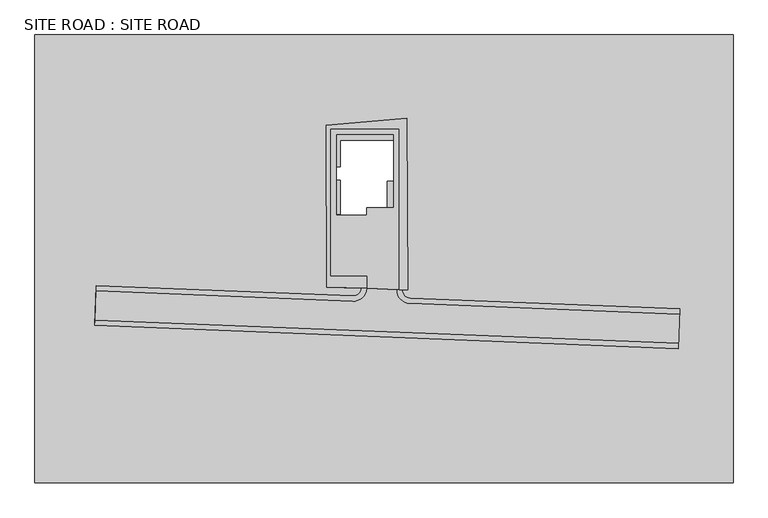
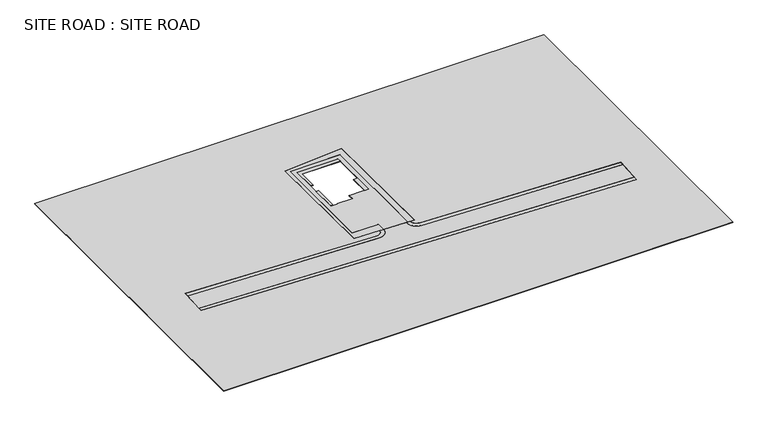
"""IFC4 building model written with IfcOpenShell, lengths in millimetres: proxy geometry, SITE ROAD : SITE ROAD."""

from ifc_helpers import new_model, si_unit, point, frame, frame_2d, origin, origin_with_axes, place, context, project, spatial, polyline, circle_curve, trimmed, segment, composite_curve, outline, extrude, source, transform, mapped, element, save


def site_road_site_road_cda8f1bc(model_context):
    return source(origin(), model_context, "Body", "SweptSolid", [
        extrude(outline(composite_curve([segment(polyline([(-5323.4846863, -24160.3398157), (379.8530763, -24364.5268641)]), True, "CONTINUOUS"), segment(trimmed(circle_curve(frame_2d((2878.0993081, -24458.1525289)), 2500.0), [point((379.8530763, -24364.5268641))], [point((2778.0134737, -26956.1482907))], True, "CARTESIAN"), True, "CONTINUOUS"), segment(polyline([(2778.0134737, -26956.1482907), (53419.5551039, -28985.1753319), (53193.7504784, -34479.8199844), (-56289.5137381, -30093.2137218), (-56064.839832, -24626.0835674), (-7921.4347509, -26555.0191334)]), True, "CONTINUOUS"), segment(trimmed(circle_curve(frame_2d((-7821.3489165, -24057.0233717)), 2500.0), [point((-7921.4347509, -26555.0191334))], [point((-5323.4846863, -24160.3398157))], True, "CARTESIAN"), True, "CONTINUOUS")], self_intersect=False)), origin_with_axes(), (0.0, 0.0, 1.0), 75.0),
        extrude(outline(polyline([(-10908.8712297, -3817.0014262), (-10308.8712297, -3817.0014262), (-10308.8712297, -10267.0014262), (-10908.8712297, -10267.0014262), (-10908.8712297, -3817.0014262)])), origin_with_axes(), (0.0, 0.0, 1.0), 100.0),
        extrude(outline(polyline([(-358.8712297, -4047.0014262), (-358.8712297, -8877.0014262), (-1448.8712297, -8877.0014262), (-1448.8712297, -4047.0014262), (-358.8712297, -4047.0014262)])), origin_with_axes(), (0.0, 0.0, 1.0), 100.0),
        extrude(outline(polyline([(-358.8712297, 3642.9985738), (-10308.8712297, 3642.9985738), (-10308.8712297, -1317.0014262), (-10908.8712297, -1317.0014262), (-10908.8712297, 4642.9985738), (-358.8712297, 4642.9985738), (-358.8712297, 3642.9985738)])), origin_with_axes(), (0.0, 0.0, 1.0), 100.0),
        extrude(outline(polyline([(-12108.8712297, 5842.9985738), (-12108.8712297, -21842.3863739), (-5323.4846863, -21842.3863739), (-5323.4846863, -24160.3398157), (-12818.4447396, -23892.0103155), (-12941.7553777, 6437.7390155), (2241.41409, 7752.6401203), (2409.7426273, -24437.1995995), (841.1287703, -24381.0411451), (841.1287703, 5842.9985738), (-12108.8712297, 5842.9985738)])), origin_with_axes(), (0.0, 0.0, 1.0), 100.0),
        extrude(outline(polyline([(63434.9499784, 23414.0184336), (63434.9499784, -60585.9815664), (-67565.0500216, -60585.9815664), (-67565.0500216, 23414.0184336), (63434.9499784, 23414.0184336)]), holes=[composite_curve([segment(polyline([(-12941.7553777, 6437.7390155), (-12818.4232308, -23897.3006555), (-6323.0723485, -24129.8428229)]), True, "CONTINUOUS"), segment(trimmed(circle_curve(frame_2d((-7821.6488643, -24064.5096292)), 1500.0), [point((-6323.0723485, -24129.8428229))], [point((-7881.7003649, -25563.3070863))], False, "CARTESIAN"), True, "CONTINUOUS"), segment(polyline([(-7881.7003649, -25563.3070863), (-56024.0812791, -23634.412555), (-56330.7861339, -31097.6528943), (53152.4780827, -35484.2591569), (53460.3136567, -27993.5043195), (2817.7478597, -25964.4362435)]), True, "CONTINUOUS"), segment(trimmed(circle_curve(frame_2d((2877.7993603, -24465.6387865)), 1500.0), [point((2817.7478597, -25964.4362435))], [point((1379.0019032, -24405.5872858))], False, "CARTESIAN"), True, "CONTINUOUS"), segment(polyline([(1379.0019032, -24405.5872858), (2409.7702929, -24442.4901599), (2241.41409, 7752.6401203), (-12941.7553777, 6437.7390155)]), True, "CONTINUOUS")], self_intersect=False)]), origin_with_axes(), (0.0, 0.0, 1.0), 125.0),
        extrude(outline(composite_curve([segment(polyline([(-26956.1482907, 2778.0134737), (-28985.1753319, 53419.5551039), (-27988.2223262, 53460.5252875), (-25959.1542503, 2817.9594904)]), True, "CONTINUOUS"), segment(trimmed(circle_curve(frame_2d((-24460.3567932, 2878.010991)), 1500.0), [point((-25959.1542503, 2817.9594904))], [point((-24400.3052926, 1379.213534))], True, "CARTESIAN"), True, "CONTINUOUS"), segment(polyline([(-24400.3052926, 1379.213534), (-24405.5872858, 1379.0019032), (-24364.5268641, 379.8530763)]), True, "CONTINUOUS"), segment(trimmed(circle_curve(frame_2d((-24458.1525289, 2878.0993081)), 2500.0), [point((-24364.5268641, 379.8530763))], [point((-26956.1482907, 2778.0134737))], False, "CARTESIAN"), True, "CONTINUOUS")], self_intersect=False)), frame((0.0, 0.0, 80.0), z_axis=(0.0, 0.0, -1.0), x_axis=(0.0, 1.0, 0.0)), (0.0, 0.0, 1.0), 80.0),
        extrude(outline(polyline([(53193.7504784, -34479.8199844), (53152.6897134, -35478.9771636), (-56330.5745031, -31092.3709011), (-56289.5137381, -30093.2137218), (53193.7504784, -34479.8199844)])), origin_with_axes(), (0.0, 0.0, 1.0), 80.0),
        extrude(outline(composite_curve([segment(polyline([(-56064.839832, -24626.0835674), (-56023.8696484, -23629.1305617), (-7881.4887342, -25558.025093)]), True, "CONTINUOUS"), segment(trimmed(circle_curve(frame_2d((-7821.4372335, -24059.2276359)), 1500.0), [point((-7881.4887342, -25558.025093))], [point((-6322.6397765, -24119.2791366))], True, "CARTESIAN"), True, "CONTINUOUS"), segment(polyline([(-6322.6397765, -24119.2791366), (-5323.4846863, -24160.3398157)]), True, "CONTINUOUS"), segment(trimmed(circle_curve(frame_2d((-7821.3489165, -24057.0233717)), 2500.0), [point((-5323.4846863, -24160.3398157))], [point((-7921.4347509, -26555.0191334))], False, "CARTESIAN"), True, "CONTINUOUS"), segment(polyline([(-7921.4347509, -26555.0191334), (-56064.839832, -24626.0835674)]), True, "CONTINUOUS")], self_intersect=False)), origin_with_axes(), (0.0, 0.0, 1.0), 80.0),
        extrude(outline(polyline([(841.1287703, 5842.9985738), (841.1287703, -24381.0411451), (-5323.4846863, -24160.3398157), (-5323.4846863, -21842.3863739), (-12108.8712297, -21842.3863739), (-12108.8712297, 5842.9985738), (841.1287703, 5842.9985738)]), holes=[polyline([(-1653.4846863, -8877.0014262), (-358.8712297, -8877.0014262), (-358.8712297, 4642.9985738), (-10513.4846863, 4642.9985738), (-10908.8712297, 4642.9985738), (-10908.8712297, -567.3863739), (-10908.8712297, -10317.0014262), (-9308.1448516, -10317.0014262), (-9283.1448516, -10292.0014262), (-5736.5057893, -10292.0014262), (-5711.5057893, -10317.0014262), (-5348.8712297, -10317.0014262), (-5348.8712297, -8877.0014262), (-1653.4846863, -8877.0014262)])]), origin_with_axes(), (0.0, 0.0, 1.0), 75.0),
    ])


if __name__ == "__main__":
    model = new_model("IFC4")
    model_context = context("Model", 3, world=origin())
    ifc_project = project(units=[si_unit("LENGTHUNIT", "METRE", prefix="MILLI")], contexts=[model_context])
    site = spatial("IfcSite", under=ifc_project)
    building = spatial("IfcBuilding", under=site)
    placement = place(None, origin())
    site_road_site_road_shape = site_road_site_road_cda8f1bc(model_context)
    element("IfcBuildingElementProxy", 1, Name="SITE ROAD : SITE ROAD", ObjectType="SITE ROAD : SITE ROAD", at=placement, inside=building, context=model_context, shape_type="MappedRepresentation", body=[
        mapped(site_road_site_road_shape, transform((0.0, 0.0, 0.0), x_axis=(1.0, 0.0, 0.0), y_axis=(0.0, 1.0, 0.0), z_axis=(0.0, 0.0, 1.0))),
    ])
    save(model, "model.ifc")

# Revit data of these elements
# Element 1 (IfcBuildingElementProxy, "SITE ROAD : SITE ROAD")
#   Materials on its faces: "Grass 02", "Pavement 13, Herringbone", "Concrete 04"
# Materials
#   "Grass 02": colour RGB 100 122 63, transparency 0, Cost = 0
#   "Pavement 13, Herringbone": colour RGB 134 134 134, transparency 0, Cost = 0
#   "Concrete 04": colour RGB 80 80 80, transparency 0
